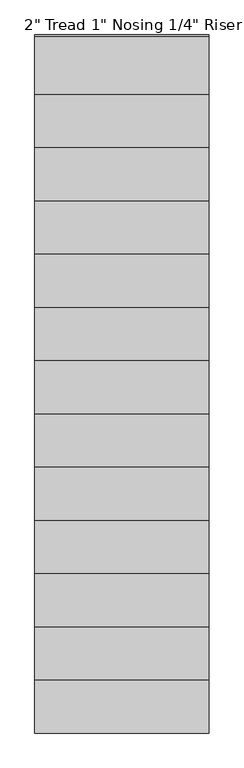
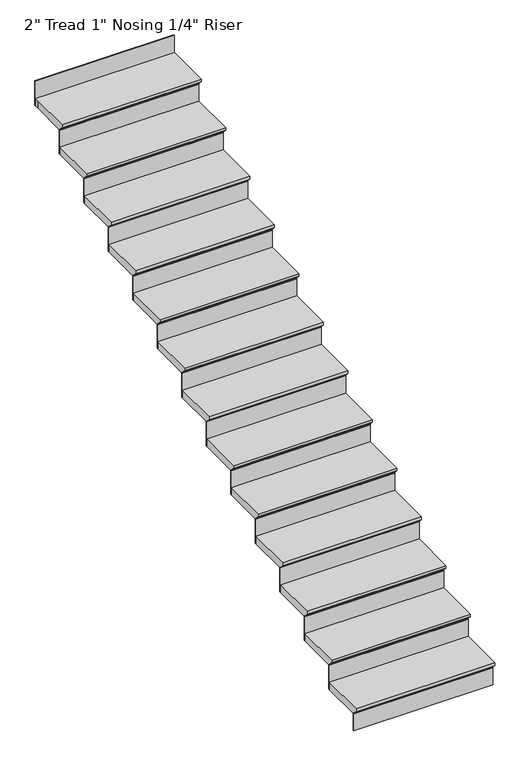
"""IFC4 building model written with IfcOpenShell, lengths in millimetres: stair flight geometry."""

from ifc_helpers import new_model, si_unit, origin, place, context, project, spatial, faceted_brep, source, transform, mapped, element, save


def stair_flight_fa816d22(model_context):
    return source(origin(), model_context, "Body", "Brep", [
        faceted_brep([(-2703.0415084, -23154.3851539, 31480.9005799), (-2703.0415084, -23154.3851539, 31499.9505799), (-3617.4415084, -23154.3851539, 31499.9505799), (-3617.4415084, -23154.3851539, 31480.9005799), (-2703.0415084, -23128.9851539, 31455.5005799), (-3617.4415084, -23128.9851539, 31455.5005799), (-2703.0415084, -22849.5851539, 31499.9505799), (-3617.4415084, -22849.5851539, 31499.9505799), (-3617.4415084, -23128.9851539, 31449.1505799), (-3617.4415084, -22849.5851539, 31449.1505799), (-2703.0415084, -22849.5851539, 31449.1505799), (-2703.0415084, -23128.9851539, 31449.1505799)], [[[0, 1, 2, 3]], [[4, 0, 3, 5]], [[2, 1, 6, 7]], [[8, 9, 10, 11]], [[2, 7, 9, 8, 5, 3]], [[8, 11, 4, 5]], [[6, 1, 0, 4, 11, 10]], [[7, 6, 10, 9]]]),
        faceted_brep([(-2703.0415084, -23128.9851539, 31449.1505799), (-2703.0415084, -23128.9851539, 31330.6172466), (-2703.0415084, -23122.6351539, 31330.6172466), (-2703.0415084, -23122.6351539, 31449.1505799), (-3617.4415084, -23128.9851539, 31449.1505799), (-3617.4415084, -23122.6351539, 31449.1505799), (-3617.4415084, -23122.6351539, 31330.6172466), (-3617.4415084, -23128.9851539, 31330.6172466)], [[[0, 1, 2, 3]], [[4, 5, 6, 7]], [[1, 0, 4, 7]], [[2, 1, 7, 6]], [[3, 2, 6, 5]], [[0, 3, 5, 4]]]),
        faceted_brep([(-2703.0415084, -22849.5851539, 31618.4839133), (-2703.0415084, -22849.5851539, 31449.1505799), (-2703.0415084, -22843.2351539, 31449.1505799), (-2703.0415084, -22843.2351539, 31618.4839133), (-3617.4415084, -22849.5851539, 31618.4839133), (-3617.4415084, -22843.2351539, 31618.4839133), (-3617.4415084, -22843.2351539, 31449.1505799), (-3617.4415084, -22849.5851539, 31449.1505799)], [[[0, 1, 2, 3]], [[4, 5, 6, 7]], [[1, 0, 4, 7]], [[2, 1, 7, 6]], [[3, 2, 6, 5]], [[0, 3, 5, 4]]]),
        faceted_brep([(-3617.4415084, -22874.9851539, 31669.2839133), (-2703.0415084, -22874.9851539, 31669.2839133), (-2703.0415084, -22570.1851539, 31669.2839133), (-3617.4415084, -22570.1851539, 31669.2839133), (-3617.4415084, -22849.5851539, 31618.4839133), (-3617.4415084, -22570.1851539, 31618.4839133), (-2703.0415084, -22570.1851539, 31618.4839133), (-2703.0415084, -22849.5851539, 31618.4839133), (-3617.4415084, -22849.5851539, 31624.8339133), (-3617.4415084, -22874.9851539, 31650.2339133), (-2703.0415084, -22849.5851539, 31624.8339133), (-2703.0415084, -22874.9851539, 31650.2339133)], [[[0, 1, 2, 3]], [[4, 5, 6, 7]], [[0, 3, 5, 4, 8, 9]], [[4, 7, 10, 8]], [[2, 1, 11, 10, 7, 6]], [[3, 2, 6, 5]], [[11, 1, 0, 9]], [[10, 11, 9, 8]]]),
        faceted_brep([(-2703.0415084, -22570.1851539, 31787.8172466), (-2703.0415084, -22570.1851539, 31618.4839133), (-2703.0415084, -22563.8351539, 31618.4839133), (-2703.0415084, -22563.8351539, 31787.8172466), (-3617.4415084, -22570.1851539, 31787.8172466), (-3617.4415084, -22563.8351539, 31787.8172466), (-3617.4415084, -22563.8351539, 31618.4839133), (-3617.4415084, -22570.1851539, 31618.4839133)], [[[0, 1, 2, 3]], [[4, 5, 6, 7]], [[1, 0, 4, 7]], [[2, 1, 7, 6]], [[3, 2, 6, 5]], [[0, 3, 5, 4]]]),
        faceted_brep([(-3617.4415084, -22595.5851539, 31838.6172466), (-2703.0415084, -22595.5851539, 31838.6172466), (-2703.0415084, -22290.7851539, 31838.6172466), (-3617.4415084, -22290.7851539, 31838.6172466), (-3617.4415084, -22570.1851539, 31787.8172466), (-3617.4415084, -22290.7851539, 31787.8172466), (-2703.0415084, -22290.7851539, 31787.8172466), (-2703.0415084, -22570.1851539, 31787.8172466), (-3617.4415084, -22570.1851539, 31794.1672466), (-3617.4415084, -22595.5851539, 31819.5672466), (-2703.0415084, -22570.1851539, 31794.1672466), (-2703.0415084, -22595.5851539, 31819.5672466)], [[[0, 1, 2, 3]], [[4, 5, 6, 7]], [[0, 3, 5, 4, 8, 9]], [[4, 7, 10, 8]], [[2, 1, 11, 10, 7, 6]], [[3, 2, 6, 5]], [[11, 1, 0, 9]], [[10, 11, 9, 8]]]),
        faceted_brep([(-2703.0415084, -22290.7851539, 31957.1505799), (-2703.0415084, -22290.7851539, 31787.8172466), (-2703.0415084, -22284.4351539, 31787.8172466), (-2703.0415084, -22284.4351539, 31957.1505799), (-3617.4415084, -22290.7851539, 31957.1505799), (-3617.4415084, -22284.4351539, 31957.1505799), (-3617.4415084, -22284.4351539, 31787.8172466), (-3617.4415084, -22290.7851539, 31787.8172466)], [[[0, 1, 2, 3]], [[4, 5, 6, 7]], [[1, 0, 4, 7]], [[2, 1, 7, 6]], [[3, 2, 6, 5]], [[0, 3, 5, 4]]]),
        faceted_brep([(-3617.4415084, -22316.1851539, 32007.9505799), (-2703.0415084, -22316.1851539, 32007.9505799), (-2703.0415084, -22011.3851539, 32007.9505799), (-3617.4415084, -22011.3851539, 32007.9505799), (-3617.4415084, -22290.7851539, 31957.1505799), (-3617.4415084, -22011.3851539, 31957.1505799), (-2703.0415084, -22011.3851539, 31957.1505799), (-2703.0415084, -22290.7851539, 31957.1505799), (-3617.4415084, -22290.7851539, 31963.5005799), (-3617.4415084, -22316.1851539, 31988.9005799), (-2703.0415084, -22290.7851539, 31963.5005799), (-2703.0415084, -22316.1851539, 31988.9005799)], [[[0, 1, 2, 3]], [[4, 5, 6, 7]], [[0, 3, 5, 4, 8, 9]], [[4, 7, 10, 8]], [[2, 1, 11, 10, 7, 6]], [[3, 2, 6, 5]], [[11, 1, 0, 9]], [[10, 11, 9, 8]]]),
        faceted_brep([(-2703.0415084, -22011.3851539, 32126.4839133), (-2703.0415084, -22011.3851539, 31957.1505799), (-2703.0415084, -22005.0351539, 31957.1505799), (-2703.0415084, -22005.0351539, 32126.4839133), (-3617.4415084, -22011.3851539, 32126.4839133), (-3617.4415084, -22005.0351539, 32126.4839133), (-3617.4415084, -22005.0351539, 31957.1505799), (-3617.4415084, -22011.3851539, 31957.1505799)], [[[0, 1, 2, 3]], [[4, 5, 6, 7]], [[1, 0, 4, 7]], [[2, 1, 7, 6]], [[3, 2, 6, 5]], [[0, 3, 5, 4]]]),
        faceted_brep([(-3617.4415084, -22036.7851539, 32177.2839133), (-2703.0415084, -22036.7851539, 32177.2839133), (-2703.0415084, -21731.9851539, 32177.2839133), (-3617.4415084, -21731.9851539, 32177.2839133), (-3617.4415084, -22011.3851539, 32126.4839133), (-3617.4415084, -21731.9851539, 32126.4839133), (-2703.0415084, -21731.9851539, 32126.4839133), (-2703.0415084, -22011.3851539, 32126.4839133), (-3617.4415084, -22011.3851539, 32132.8339133), (-3617.4415084, -22036.7851539, 32158.2339133), (-2703.0415084, -22011.3851539, 32132.8339133), (-2703.0415084, -22036.7851539, 32158.2339133)], [[[0, 1, 2, 3]], [[4, 5, 6, 7]], [[0, 3, 5, 4, 8, 9]], [[4, 7, 10, 8]], [[2, 1, 11, 10, 7, 6]], [[3, 2, 6, 5]], [[11, 1, 0, 9]], [[10, 11, 9, 8]]]),
        faceted_brep([(-2703.0415084, -21731.9851539, 32295.8172466), (-2703.0415084, -21731.9851539, 32126.4839133), (-2703.0415084, -21725.6351539, 32126.4839133), (-2703.0415084, -21725.6351539, 32295.8172466), (-3617.4415084, -21731.9851539, 32295.8172466), (-3617.4415084, -21725.6351539, 32295.8172466), (-3617.4415084, -21725.6351539, 32126.4839133), (-3617.4415084, -21731.9851539, 32126.4839133)], [[[0, 1, 2, 3]], [[4, 5, 6, 7]], [[1, 0, 4, 7]], [[2, 1, 7, 6]], [[3, 2, 6, 5]], [[0, 3, 5, 4]]]),
        faceted_brep([(-3617.4415084, -21757.3851539, 32346.6172466), (-2703.0415084, -21757.3851539, 32346.6172466), (-2703.0415084, -21452.5851539, 32346.6172466), (-3617.4415084, -21452.5851539, 32346.6172466), (-3617.4415084, -21731.9851539, 32295.8172466), (-3617.4415084, -21452.5851539, 32295.8172466), (-2703.0415084, -21452.5851539, 32295.8172466), (-2703.0415084, -21731.9851539, 32295.8172466), (-3617.4415084, -21731.9851539, 32302.1672466), (-3617.4415084, -21757.3851539, 32327.5672466), (-2703.0415084, -21731.9851539, 32302.1672466), (-2703.0415084, -21757.3851539, 32327.5672466)], [[[0, 1, 2, 3]], [[4, 5, 6, 7]], [[0, 3, 5, 4, 8, 9]], [[4, 7, 10, 8]], [[2, 1, 11, 10, 7, 6]], [[3, 2, 6, 5]], [[11, 1, 0, 9]], [[10, 11, 9, 8]]]),
        faceted_brep([(-2703.0415084, -21452.5851539, 32465.1505799), (-2703.0415084, -21452.5851539, 32295.8172466), (-2703.0415084, -21446.2351539, 32295.8172466), (-2703.0415084, -21446.2351539, 32465.1505799), (-3617.4415084, -21452.5851539, 32465.1505799), (-3617.4415084, -21446.2351539, 32465.1505799), (-3617.4415084, -21446.2351539, 32295.8172466), (-3617.4415084, -21452.5851539, 32295.8172466)], [[[0, 1, 2, 3]], [[4, 5, 6, 7]], [[1, 0, 4, 7]], [[2, 1, 7, 6]], [[3, 2, 6, 5]], [[0, 3, 5, 4]]]),
        faceted_brep([(-3617.4415084, -21477.9851539, 32515.9505799), (-2703.0415084, -21477.9851539, 32515.9505799), (-2703.0415084, -21173.1851539, 32515.9505799), (-3617.4415084, -21173.1851539, 32515.9505799), (-3617.4415084, -21452.5851539, 32465.1505799), (-3617.4415084, -21173.1851539, 32465.1505799), (-2703.0415084, -21173.1851539, 32465.1505799), (-2703.0415084, -21452.5851539, 32465.1505799), (-3617.4415084, -21452.5851539, 32471.5005799), (-3617.4415084, -21477.9851539, 32496.9005799), (-2703.0415084, -21452.5851539, 32471.5005799), (-2703.0415084, -21477.9851539, 32496.9005799)], [[[0, 1, 2, 3]], [[4, 5, 6, 7]], [[0, 3, 5, 4, 8, 9]], [[4, 7, 10, 8]], [[2, 1, 11, 10, 7, 6]], [[3, 2, 6, 5]], [[11, 1, 0, 9]], [[10, 11, 9, 8]]]),
        faceted_brep([(-2703.0415084, -21173.1851539, 32634.4839133), (-2703.0415084, -21173.1851539, 32465.1505799), (-2703.0415084, -21166.8351539, 32465.1505799), (-2703.0415084, -21166.8351539, 32634.4839133), (-3617.4415084, -21173.1851539, 32634.4839133), (-3617.4415084, -21166.8351539, 32634.4839133), (-3617.4415084, -21166.8351539, 32465.1505799), (-3617.4415084, -21173.1851539, 32465.1505799)], [[[0, 1, 2, 3]], [[4, 5, 6, 7]], [[1, 0, 4, 7]], [[2, 1, 7, 6]], [[3, 2, 6, 5]], [[0, 3, 5, 4]]]),
        faceted_brep([(-3617.4415084, -21198.5851539, 32685.2839133), (-2703.0415084, -21198.5851539, 32685.2839133), (-2703.0415084, -20893.7851539, 32685.2839133), (-3617.4415084, -20893.7851539, 32685.2839133), (-3617.4415084, -21173.1851539, 32634.4839133), (-3617.4415084, -20893.7851539, 32634.4839133), (-2703.0415084, -20893.7851539, 32634.4839133), (-2703.0415084, -21173.1851539, 32634.4839133), (-3617.4415084, -21173.1851539, 32640.8339133), (-3617.4415084, -21198.5851539, 32666.2339133), (-2703.0415084, -21173.1851539, 32640.8339133), (-2703.0415084, -21198.5851539, 32666.2339133)], [[[0, 1, 2, 3]], [[4, 5, 6, 7]], [[0, 3, 5, 4, 8, 9]], [[4, 7, 10, 8]], [[2, 1, 11, 10, 7, 6]], [[3, 2, 6, 5]], [[11, 1, 0, 9]], [[10, 11, 9, 8]]]),
        faceted_brep([(-2703.0415084, -20893.7851539, 32803.8172466), (-2703.0415084, -20893.7851539, 32634.4839133), (-2703.0415084, -20887.4351539, 32634.4839133), (-2703.0415084, -20887.4351539, 32803.8172466), (-3617.4415084, -20893.7851539, 32803.8172466), (-3617.4415084, -20887.4351539, 32803.8172466), (-3617.4415084, -20887.4351539, 32634.4839133), (-3617.4415084, -20893.7851539, 32634.4839133)], [[[0, 1, 2, 3]], [[4, 5, 6, 7]], [[1, 0, 4, 7]], [[2, 1, 7, 6]], [[3, 2, 6, 5]], [[0, 3, 5, 4]]]),
        faceted_brep([(-3617.4415084, -20919.1851539, 32854.6172466), (-2703.0415084, -20919.1851539, 32854.6172466), (-2703.0415084, -20614.3851539, 32854.6172466), (-3617.4415084, -20614.3851539, 32854.6172466), (-3617.4415084, -20893.7851539, 32803.8172466), (-3617.4415084, -20614.3851539, 32803.8172466), (-2703.0415084, -20614.3851539, 32803.8172466), (-2703.0415084, -20893.7851539, 32803.8172466), (-3617.4415084, -20893.7851539, 32810.1672466), (-3617.4415084, -20919.1851539, 32835.5672466), (-2703.0415084, -20893.7851539, 32810.1672466), (-2703.0415084, -20919.1851539, 32835.5672466)], [[[0, 1, 2, 3]], [[4, 5, 6, 7]], [[0, 3, 5, 4, 8, 9]], [[4, 7, 10, 8]], [[2, 1, 11, 10, 7, 6]], [[3, 2, 6, 5]], [[11, 1, 0, 9]], [[10, 11, 9, 8]]]),
        faceted_brep([(-2703.0415084, -20614.3851539, 32973.1505799), (-2703.0415084, -20614.3851539, 32803.8172466), (-2703.0415084, -20608.0351539, 32803.8172466), (-2703.0415084, -20608.0351539, 32973.1505799), (-3617.4415084, -20614.3851539, 32973.1505799), (-3617.4415084, -20608.0351539, 32973.1505799), (-3617.4415084, -20608.0351539, 32803.8172466), (-3617.4415084, -20614.3851539, 32803.8172466)], [[[0, 1, 2, 3]], [[4, 5, 6, 7]], [[1, 0, 4, 7]], [[2, 1, 7, 6]], [[3, 2, 6, 5]], [[0, 3, 5, 4]]]),
        faceted_brep([(-3617.4415084, -20639.7851539, 33023.9505799), (-2703.0415084, -20639.7851539, 33023.9505799), (-2703.0415084, -20334.9851539, 33023.9505799), (-3617.4415084, -20334.9851539, 33023.9505799), (-3617.4415084, -20614.3851539, 32973.1505799), (-3617.4415084, -20334.9851539, 32973.1505799), (-2703.0415084, -20334.9851539, 32973.1505799), (-2703.0415084, -20614.3851539, 32973.1505799), (-3617.4415084, -20614.3851539, 32979.5005799), (-3617.4415084, -20639.7851539, 33004.9005799), (-2703.0415084, -20614.3851539, 32979.5005799), (-2703.0415084, -20639.7851539, 33004.9005799)], [[[0, 1, 2, 3]], [[4, 5, 6, 7]], [[0, 3, 5, 4, 8, 9]], [[4, 7, 10, 8]], [[2, 1, 11, 10, 7, 6]], [[3, 2, 6, 5]], [[11, 1, 0, 9]], [[10, 11, 9, 8]]]),
        faceted_brep([(-2703.0415084, -20334.9851539, 33142.4839133), (-2703.0415084, -20334.9851539, 32973.1505799), (-2703.0415084, -20328.6351539, 32973.1505799), (-2703.0415084, -20328.6351539, 33142.4839133), (-3617.4415084, -20334.9851539, 33142.4839133), (-3617.4415084, -20328.6351539, 33142.4839133), (-3617.4415084, -20328.6351539, 32973.1505799), (-3617.4415084, -20334.9851539, 32973.1505799)], [[[0, 1, 2, 3]], [[4, 5, 6, 7]], [[1, 0, 4, 7]], [[2, 1, 7, 6]], [[3, 2, 6, 5]], [[0, 3, 5, 4]]]),
        faceted_brep([(-3617.4415084, -20360.3851539, 33193.2839133), (-2703.0415084, -20360.3851539, 33193.2839133), (-2703.0415084, -20055.5851539, 33193.2839133), (-3617.4415084, -20055.5851539, 33193.2839133), (-3617.4415084, -20334.9851539, 33142.4839133), (-3617.4415084, -20055.5851539, 33142.4839133), (-2703.0415084, -20055.5851539, 33142.4839133), (-2703.0415084, -20334.9851539, 33142.4839133), (-3617.4415084, -20334.9851539, 33148.8339133), (-3617.4415084, -20360.3851539, 33174.2339133), (-2703.0415084, -20334.9851539, 33148.8339133), (-2703.0415084, -20360.3851539, 33174.2339133)], [[[0, 1, 2, 3]], [[4, 5, 6, 7]], [[0, 3, 5, 4, 8, 9]], [[4, 7, 10, 8]], [[2, 1, 11, 10, 7, 6]], [[3, 2, 6, 5]], [[11, 1, 0, 9]], [[10, 11, 9, 8]]]),
        faceted_brep([(-2703.0415084, -20055.5851539, 33311.8172466), (-2703.0415084, -20055.5851539, 33142.4839133), (-2703.0415084, -20049.2351539, 33142.4839133), (-2703.0415084, -20049.2351539, 33311.8172466), (-3617.4415084, -20055.5851539, 33311.8172466), (-3617.4415084, -20049.2351539, 33311.8172466), (-3617.4415084, -20049.2351539, 33142.4839133), (-3617.4415084, -20055.5851539, 33142.4839133)], [[[0, 1, 2, 3]], [[4, 5, 6, 7]], [[1, 0, 4, 7]], [[2, 1, 7, 6]], [[3, 2, 6, 5]], [[0, 3, 5, 4]]]),
        faceted_brep([(-3617.4415084, -20080.9851539, 33362.6172466), (-2703.0415084, -20080.9851539, 33362.6172466), (-2703.0415084, -19776.1851539, 33362.6172466), (-3617.4415084, -19776.1851539, 33362.6172466), (-3617.4415084, -20055.5851539, 33311.8172466), (-3617.4415084, -19776.1851539, 33311.8172466), (-2703.0415084, -19776.1851539, 33311.8172466), (-2703.0415084, -20055.5851539, 33311.8172466), (-3617.4415084, -20055.5851539, 33318.1672466), (-3617.4415084, -20080.9851539, 33343.5672466), (-2703.0415084, -20055.5851539, 33318.1672466), (-2703.0415084, -20080.9851539, 33343.5672466)], [[[0, 1, 2, 3]], [[4, 5, 6, 7]], [[0, 3, 5, 4, 8, 9]], [[4, 7, 10, 8]], [[2, 1, 11, 10, 7, 6]], [[3, 2, 6, 5]], [[11, 1, 0, 9]], [[10, 11, 9, 8]]]),
        faceted_brep([(-2703.0415084, -19496.7851539, 33650.4839133), (-2703.0415084, -19496.7851539, 33481.1505799), (-2703.0415084, -19490.4351539, 33481.1505799), (-2703.0415084, -19490.4351539, 33650.4839133), (-3617.4415084, -19496.7851539, 33650.4839133), (-3617.4415084, -19490.4351539, 33650.4839133), (-3617.4415084, -19490.4351539, 33481.1505799), (-3617.4415084, -19496.7851539, 33481.1505799)], [[[0, 1, 2, 3]], [[4, 5, 6, 7]], [[1, 0, 4, 7]], [[2, 1, 7, 6]], [[3, 2, 6, 5]], [[0, 3, 5, 4]]]),
        faceted_brep([(-2703.0415084, -19776.1851539, 33481.1505799), (-2703.0415084, -19776.1851539, 33311.8172466), (-2703.0415084, -19769.8351539, 33311.8172466), (-2703.0415084, -19769.8351539, 33481.1505799), (-3617.4415084, -19776.1851539, 33481.1505799), (-3617.4415084, -19769.8351539, 33481.1505799), (-3617.4415084, -19769.8351539, 33311.8172466), (-3617.4415084, -19776.1851539, 33311.8172466)], [[[0, 1, 2, 3]], [[4, 5, 6, 7]], [[1, 0, 4, 7]], [[2, 1, 7, 6]], [[3, 2, 6, 5]], [[0, 3, 5, 4]]]),
        faceted_brep([(-3617.4415084, -19496.7851539, 33531.9505799), (-3617.4415084, -19522.1851539, 33531.9505799), (-3617.4415084, -19801.5851539, 33531.9505799), (-2703.0415084, -19801.5851539, 33531.9505799), (-2703.0415084, -19496.7851539, 33531.9505799), (-3617.4415084, -19522.1851539, 33481.1505799), (-3617.4415084, -19496.7851539, 33481.1505799), (-2703.0415084, -19496.7851539, 33481.1505799), (-2703.0415084, -19776.1851539, 33481.1505799), (-3617.4415084, -19776.1851539, 33481.1505799), (-3617.4415084, -19776.1851539, 33487.5005799), (-3617.4415084, -19801.5851539, 33512.9005799), (-2703.0415084, -19776.1851539, 33487.5005799), (-2703.0415084, -19801.5851539, 33512.9005799)], [[[0, 1, 2, 3, 4]], [[5, 6, 7, 8, 9]], [[1, 0, 6, 5]], [[2, 1, 5, 9, 10, 11]], [[9, 8, 12, 10]], [[4, 3, 13, 12, 8, 7]], [[0, 4, 7, 6]], [[13, 3, 2, 11]], [[12, 13, 11, 10]]]),
    ])


if __name__ == "__main__":
    model = new_model("IFC4")
    model_context = context("Model", 3, world=origin())
    ifc_project = project(units=[si_unit("LENGTHUNIT", "METRE", prefix="MILLI")], contexts=[model_context])
    site = spatial("IfcSite", under=ifc_project)
    building = spatial("IfcBuilding", under=site)
    placement = place(None, origin())
    stair_flight_shape = stair_flight_fa816d22(model_context)
    element("IfcStairFlight", 1, ObjectType="2\" Tread 1\" Nosing 1/4\" Riser", at=placement, inside=building, context=model_context, shape_type="MappedRepresentation", body=[
        mapped(stair_flight_shape, transform((0.0, 0.0, 0.0), x_axis=(1.0, 0.0, 0.0), y_axis=(0.0, 1.0, 0.0), z_axis=(0.0, 0.0, 1.0))),
    ])
    save(model, "model.ifc")
